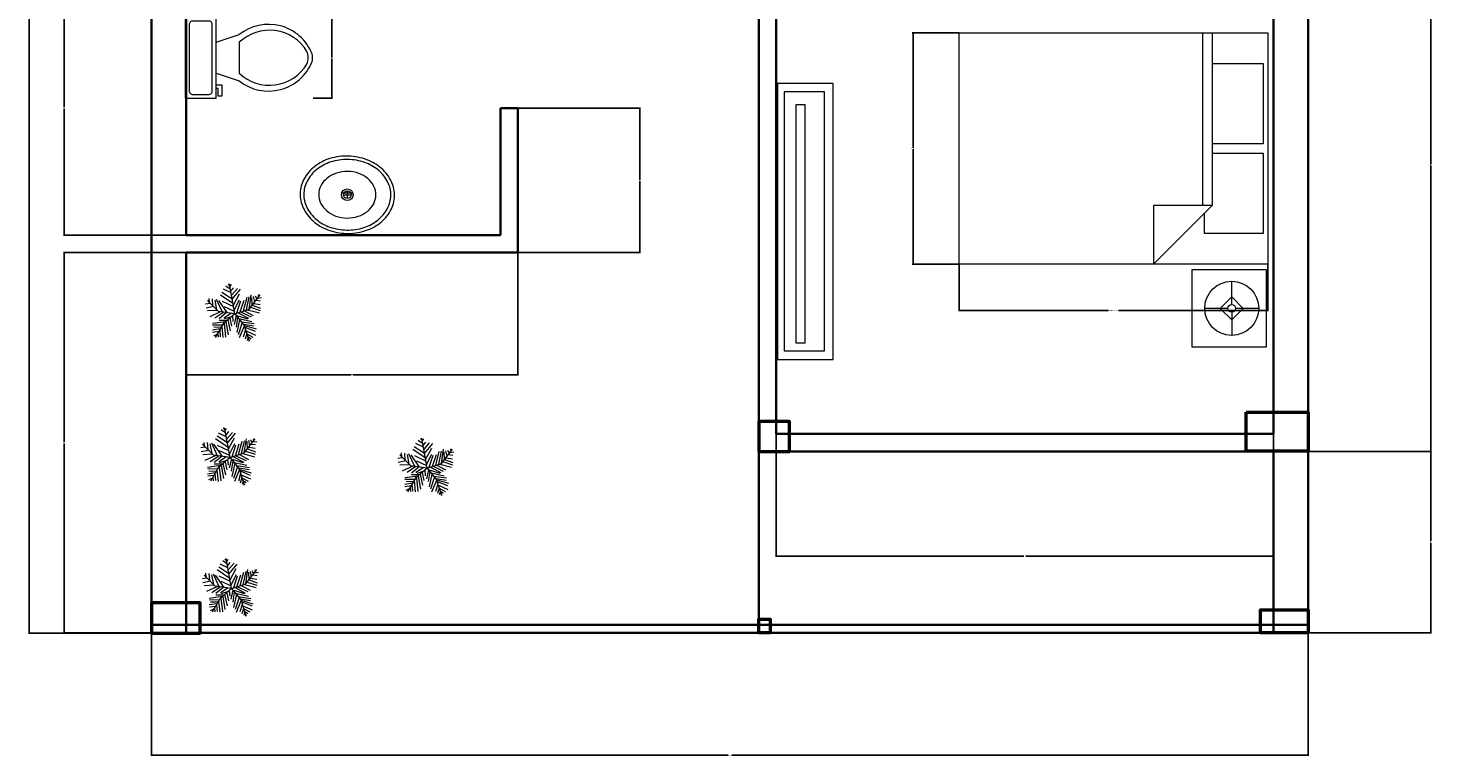
# Model space of a CAD drawing. Units: inches. Extents: x 50 to 2003, y -28 to 675.
# Tile 5 of 10: x 592 to 956, y -28 to 160. Entities that reach past the tile are written whole.
import ezdxf

# ---------------------------------------------------------------- set-up
doc = ezdxf.new("R2010")
doc.units = ezdxf.units.IN
for name, color, linetype, lineweight in [('A-ANNO-DIMS', 2, 'Continuous', 18), ('A-COLS', 1, 'Continuous', 50), ('A-FLOR-FIXT', 9, 'Continuous', 18), ('A-FURN', 8, 'Continuous', 18), ('A-FURN-LITE', 9, 'Continuous', 13), ('A-WALL', 7, 'Continuous', 35), ('L-PLNT', 3, 'Continuous', 13)]:
    doc.layers.add(name, color=color, linetype=linetype, lineweight=lineweight)
doc.styles.get("Standard").update_dxf_attribs({"font": 'arial.ttf'})
doc.dimstyles.get("Standard").update_dxf_attribs({"dimtxt": 0.18, "dimasz": 0.18, "dimexe": 0.18, "dimexo": 0.0625, "dimgap": 0.09, "dimtad": 0, "dimtih": 1, "dimtoh": 1, "dimdec": 4, "dimzin": 0, "dimdsep": 46, "dimtxsty": 'Standard', "dimcen": 0.09, "dimadec": 0, "dimazin": 0, "dimtfac": 1, "dimtdec": 4, "dimtofl": 0, "dimtmove": 0, "dimatfit": 3, "dimfxl": 1, "dimtolj": 1, "dimtzin": 0, "dimarcsym": 0})

# ---------------------------------------------------------------- blocks, each defined once
blk = doc.blocks.new('*U2')
for p, q in [((-10.186, 53.64), (-13.084, 55.962)), ((0, 0), (-10.5, 57)), ((-9.099, 51.782), (-6.563, 55.962)), ((-48.585, 21.131), (-49.309, 29.026)), ((-43.513, 28.561), (-42.427, 15.558)), ((-35.544, 28.097), (-24.314, 3.947)), ((-3.665, 19.273), (-27.574, 35.527)), ((-5.114, 28.097), (-24.676, 40.636)), ((-7.288, 39.707), (-21.778, 46.673)), ((-8.737, 47.138), (-17.069, 52.711)), ((-7.65, 43.423), (-2.578, 49.46)), ((-5.839, 35.992), (4.667, 48.067)), ((-5.114, 27.632), (10.463, 46.673)), ((-2.941, 16.486), (8.652, 37.85)), ((16.259, 5.805), (23.142, 31.348)), ((22.055, 7.198), (27.489, 32.277)), ((27, 9), (48, 36)), ((27.127, 9.056), (31.112, 35.992)), ((31.836, 30.883), (32.561, 16.486)), ((35.096, 32.741), (37.27, 22.524)), ((38.719, 34.134), (41.979, 28.561)), ((43.791, 29.954), (51.036, 30.883)), ((44.153, 36.456), (45.239, 32.741)), ((-47.498, 19.737), (-55.83, 18.344)), ((-40.615, 13.7), (-55.105, 10.913)), ((-31.5, 4.5), (-52.5, 25.5)), ((-33.37, 6.269), (-52.207, 5.34)), ((-28.299, 3.483), (-47.86, -5.805)), ((-38.442, 26.239), (-34.819, 7.663)), ((-21.416, 3.018), (-38.079, -8.128)), ((0, 0), (-31.5, 4.5)), ((-14.533, 2.09), (-30.834, 25.31)), ((-15.982, 2.09), (-30.11, -9.521)), ((-24.314, 23.917), (-2.941, 13.7)), ((0, 0), (-22.5, -19.5)), ((-6.563, 1.161), (-21.416, -8.128)), ((-20.691, 13.7), (-1.129, 4.876)), ((-1.129, 6.734), (9.014, 26.704)), ((0, 0), (27, 9)), ((0, 0), (18, -22.5)), ((3.942, 1.625), (11.187, 24.381)), ((6.478, 1.625), (26.04, -8.592)), ((10.101, 3.483), (17.708, 26.239)), ((11.187, 3.483), (30.749, -5.805)), ((18.07, 5.805), (35.096, -3.483)), ((24.229, 7.663), (46.688, 1.625)), ((29.662, 12.307), (48.137, 6.269)), ((33.285, 16.486), (48.862, 10.913)), ((36.183, 19.737), (48.137, 17.88)), ((40.53, 25.775), (48.862, 24.846)), ((-17.431, -15.094), (-42.789, -18.809)), ((-24.314, -21.596), (-42.427, -22.06)), ((-26.849, -26.24), (-40.253, -25.775)), ((-22.5, -19.5), (-37.5, -45)), ((-15.257, -12.772), (-30.11, -12.772)), ((-25.038, -23.918), (-22.865, -45.281)), ((-20.691, -18.345), (-17.793, -44.352)), ((-6.563, -5.805), (-19.967, -9.985)), ((-17.069, -15.094), (-12.721, -40.172)), ((-13.446, -11.378), (-8.737, -32.741)), ((-9.461, -8.592), (-6.201, -23.453)), ((-4.752, -3.483), (-3.665, -14.629)), ((2.493, -3.019), (-1.491, -20.202)), ((1.769, -2.555), (24.229, -9.521)), ((5.029, -6.27), (2.131, -25.775)), ((9.014, -11.378), (3.58, -35.992)), ((14.085, -16.951), (6.478, -40.172)), ((7.565, -9.056), (32.198, -14.629)), ((18.07, -22.524), (8.289, -45.745)), ((12.274, -15.094), (36.907, -18.809)), ((16.259, -19.738), (36.183, -22.989)), ((18, -22.5), (27, -52.5)), ((18.433, -22.524), (40.53, -29.026)), ((19.157, -25.311), (38.719, -33.206)), ((-28.299, -29.026), (-42.789, -31.348)), ((-30.834, -34.135), (-42.427, -35.528)), ((-34.457, -39.708), (-40.978, -42.494)), ((-32.646, -36.921), (-31.921, -44.352)), ((-29.023, -30.884), (-27.936, -43.887)), ((20.244, -30.419), (15.897, -44.816)), ((22.78, -37.85), (19.519, -48.532)), ((21.331, -32.741), (39.081, -40.636)), ((22.78, -38.314), (34.372, -44.816)), ((24.591, -45.745), (23.142, -50.854)), ((24.591, -43.423), (30.749, -47.603)), ((26.764, -49.925), (28.213, -50.854))]:
    blk.add_line(p, q)
blk = doc.blocks.new('Bed - Queen')
for p, q in [((0, -80.00003), (0, 0)), ((0, 0), (59.99999, 0)), ((59.99999, 0), (59.99999, -80.00003)), ((7.99999, -1.2), (28.79998, -1.2)), ((7.99999, -14.4), (7.99999, -1.2)), ((28.79998, -1.2), (28.79998, -14.4)), ((31.19999, -1.2), (51.99999, -1.2)), ((31.19999, -14.4), (31.19999, -1.2)), ((51.99999, -1.2), (51.99999, -16.4)), ((0, -14.4), (44.8, -14.4)), ((59.99999, -29.6), (44.8, -14.4)), ((44.8, -14.4), (44.8, -29.6)), ((44.8, -16.8), (0, -16.8)), ((51.99999, -16.4), (46.79936, -16.4)), ((44.8, -29.6), (59.99999, -29.6)), ((59.99999, -80.00003), (0, -80.00003))]:
    blk.add_line(p, q)
blk = doc.blocks.new('Lamp - Table')
for p, q in [((0, 7), (0, 1)), ((-1, 0), (-7, 0)), ((0, 3), (-3, 0)), ((-3, 0), (0, -3)), ((3, 0), (0, 3)), ((0, -3), (3, 0)), ((1, 0), (7, 0)), ((0, -1), (0, -7))]:
    blk.add_line(p, q)
for radius in [7, 1]:
    blk.add_circle((0, 0), radius)
blk = doc.blocks.new('Toilet - top')
for p, q in [((9.5, -6), (9.5, -2)), ((-10, -8.5), (-8, -8.5)), ((-10, -9.5), (-10, -8.5)), ((-7, -9.5), (-10, -9.5)), ((-8, -8.5), (-8, -8)), ((-7, -8), (-7, -9.5)), ((-4, -8), (-6, -14)), ((4, -8), (6, -14)), ((4, -14), (-4, -14))]:
    blk.add_line(p, q)
blk.add_lwpolyline([(10.5, -8), (10.5, 0), (-10.5, 0), (-10.5, -8)], close=True)
for points in [[(-9.5, -2), (-9.5, -6)], [(8.5, -1), (-8.5, -1)], [(-8.5, -7), (8.5, -7)]]:
    blk.add_lwpolyline(points)
for centre, radius, start, end in [((-8.62, -1.88), 0.884, 81.8699, 188.1301), ((8.62, -1.88), 0.884, 351.8699, 98.1301), ((-8.62, -6.12), 0.884, 171.8699, 278.1301), ((8.62, -6.12), 0.884, 261.8699, 8.1301), ((3.52, -21.58), 12.17, 141.4691, 247.9714), ((4.2, -21.82), 11.33, 136.3677, 238.9468), ((-3.52, -21.58), 12.17, 292.0284, 38.5307), ((-4.2, -21.82), 11.33, 301.053, 43.6321), ((0, -27.88), 4, 245.7318, 294.2682), ((0, -29), 4, 254.8605, 285.1395)]:
    blk.add_arc(centre, radius, start, end)
blk = doc.blocks.new('Sink - Oval top')
for p, q in [((-1, 0), (1, 0)), ((0, 1), (0, -1))]:
    blk.add_line(p, q)
for points in [[(-12.23, 0.39, 0.117634), (-11.46, -3.36, 0.104469), (-8.88, -6.8, 0.090016), (-5.08, -9.07, 0.08192), (-0.32, -10.02, 0.08192), (4.49, -9.38, 0.090016), (8.42, -7.36, 0.104469), (11.22, -4.09, 0.117634), (12.23, -0.39, 0.117634), (11.46, 3.36, 0.104469), (8.88, 6.8, 0.090016), (5.08, 9.07, 0.08192), (0.32, 10.02, 0.08192), (-4.49, 9.38, 0.090016), (-8.42, 7.36, 0.104469), (-11.22, 4.09, 0.117634)], [(-11.29, 0.16, 0.118622), (-10.52, -3.25, 0.104678), (-8.07, -6.36, 0.089562), (-4.54, -8.37, 0.081185), (-0.13, -9.15, 0.081185), (4.3, -8.49, 0.089562), (7.89, -6.58, 0.104678), (10.42, -3.55, 0.118622), (11.29, -0.16, 0.118622), (10.52, 3.25, 0.104678), (8.07, 6.36, 0.089562), (4.54, 8.37, 0.081185), (0.13, 9.15, 0.081185), (-4.3, 8.49, 0.089562), (-7.89, 6.58, 0.104678), (-10.42, 3.55, 0.118622)], [(-7.42, 0.08, 0.118283), (-6.91, -2.17, 0.104607), (-5.29, -4.21, 0.089718), (-2.97, -5.53, 0.081436), (-0.07, -6.04, 0.081436), (2.84, -5.59, 0.089718), (5.2, -4.33, 0.104607), (6.86, -2.32, 0.118283), (7.42, -0.08, 0.118283), (6.91, 2.17, 0.104607), (5.29, 4.21, 0.089718), (2.97, 5.53, 0.081436), (0.07, 6.04, 0.081436), (-2.84, 5.59, 0.089718), (-5.2, 4.33, 0.104607), (-6.86, 2.32, 0.118283)]]:
    blk.add_lwpolyline(points, format="xyb", close=True)
for radius in [1.5, 1]:
    blk.add_circle((0, 0), radius)
blk = doc.blocks.new('MEDIA-CONSOLE')
for points in [[(0, 0), (71.49, 0), (71.49, 14.4), (0, 14.4)], [(2.13, 1.7), (69.3, 1.7), (69.3, 12.15), (2.13, 12.15)], [(5.56, 4.74), (67.2, 4.74), (67.2, 7.16), (5.56, 7.16)]]:
    blk.add_lwpolyline(points, close=True)
blk = doc.blocks.new('NIGHTSTAND-STANDARD')
blk.add_lwpolyline([(0, 0), (0, 20.13), (19.19, 20.13), (19.19, 0)], close=True)
blk = doc.blocks.new('*D23')
at = {"layer": 'A-ANNO-DIMS', "color": 0, "lineweight": -2, "transparency": 16777216}
for p, q in [((833.11, 99.05), (833.11, 86.94)), ((913.11, 99.05), (913.11, 86.94)), ((833.29, 87.12), (871.8, 87.12)), ((912.93, 87.12), (874.41, 87.12))]:
    blk.add_line(p, q, dxfattribs=at)
at = {"layer": 'A-ANNO-DIMS', "color": 0, "transparency": 16777216}
for points in [[(833.29, 87.15), (833.29, 87.09), (833.11, 87.12)], [(912.93, 87.15), (912.93, 87.09), (913.11, 87.12)]]:
    blk.add_solid(points, dxfattribs=at)
at = {"layer": 'Defpoints', "color": 0, "transparency": 16777216}
for p in [(833.11, 99.12), (913.11, 99.12), (913.11, 87.12)]:
    blk.add_point(p, dxfattribs=at)
at = {"layer": 'A-ANNO-DIMS', "color": 0, "transparency": 16777216, "insert": (873.11, 87.12), "char_height": 0.18, "attachment_point": 5}
blk.add_mtext('\\A1;QUEEN BED 80 TYP.', dxfattribs=at)
blk = doc.blocks.new('*D24')
at = {"layer": 'A-ANNO-DIMS', "color": 0, "lineweight": -2, "transparency": 16777216}
for p, q in [((833.04, 159.12), (820.93, 159.12)), ((821.11, 158.94), (821.11, 129.3)), ((821.11, 99.3), (821.11, 128.93)), ((833.04, 99.12), (820.93, 99.12))]:
    blk.add_line(p, q, dxfattribs=at)
at = {"layer": 'A-ANNO-DIMS', "color": 0, "transparency": 16777216}
for points in [[(821.08, 158.94), (821.14, 158.94), (821.11, 159.12)], [(821.08, 99.3), (821.14, 99.3), (821.11, 99.12)]]:
    blk.add_solid(points, dxfattribs=at)
at = {"layer": 'Defpoints', "color": 0, "transparency": 16777216}
for p in [(833.11, 159.12), (821.11, 99.12), (833.11, 99.12)]:
    blk.add_point(p, dxfattribs=at)
at = {"layer": 'A-ANNO-DIMS', "color": 0, "transparency": 16777216, "insert": (821.11, 129.12), "char_height": 0.18, "attachment_point": 5}
blk.add_mtext('\\A1;60 TYP.', dxfattribs=at)
blk = doc.blocks.new('*D30')
at = {"layer": 'A-ANNO-DIMS', "color": 0, "lineweight": -2, "transparency": 16777216}
for p, q in [((665.51, 163.13), (670.58, 163.13)), ((670.4, 162.95), (670.4, 152.81)), ((670.4, 142.31), (670.4, 152.45)), ((665.51, 142.13), (670.58, 142.13))]:
    blk.add_line(p, q, dxfattribs=at)
at = {"layer": 'A-ANNO-DIMS', "color": 0, "transparency": 16777216}
for points in [[(670.37, 162.95), (670.43, 162.95), (670.4, 163.13)], [(670.37, 142.31), (670.43, 142.31), (670.4, 142.13)]]:
    blk.add_solid(points, dxfattribs=at)
at = {"layer": 'Defpoints', "color": 0, "transparency": 16777216}
for p in [(665.44, 163.13), (670.4, 163.13), (665.44, 142.13)]:
    blk.add_point(p, dxfattribs=at)
at = {"layer": 'A-ANNO-DIMS', "color": 0, "transparency": 16777216, "insert": (670.4, 152.63), "char_height": 0.18, "attachment_point": 5}
blk.add_mtext('\\A1;21 TYP.', dxfattribs=at)
blk = doc.blocks.new('*D74')
at = {"layer": 'A-ANNO-DIMS', "color": 0, "lineweight": -2, "transparency": 16777216}
for p, q in [((623.65, 3.46), (623.65, -28.31)), ((923.6, 3.56), (923.6, -28.31)), ((623.83, -28.13), (773.16, -28.13)), ((923.42, -28.13), (774.09, -28.13))]:
    blk.add_line(p, q, dxfattribs=at)
at = {"layer": 'A-ANNO-DIMS', "color": 0, "transparency": 16777216}
for points in [[(623.83, -28.1), (623.83, -28.16), (623.65, -28.13)], [(923.42, -28.1), (923.42, -28.16), (923.6, -28.13)]]:
    blk.add_solid(points, dxfattribs=at)
at = {"layer": 'Defpoints', "color": 0, "transparency": 16777216}
for p in [(623.65, 3.52), (923.6, 3.62), (923.6, -28.13)]:
    blk.add_point(p, dxfattribs=at)
at = {"layer": 'A-ANNO-DIMS', "color": 0, "transparency": 16777216, "insert": (773.63, -28.13), "char_height": 0.18, "attachment_point": 5}
blk.add_mtext('\\A1;299.95', dxfattribs=at)
blk = doc.blocks.new('*D75')
at = {"layer": 'A-ANNO-DIMS', "color": 0, "lineweight": -2, "transparency": 16777216}
for p, q in [((623.55, 618.62), (591.74, 618.62)), ((591.92, 618.44), (591.92, 311.25)), ((591.92, 3.7), (591.92, 310.89)), ((623.59, 3.52), (591.74, 3.52))]:
    blk.add_line(p, q, dxfattribs=at)
at = {"layer": 'A-ANNO-DIMS', "color": 0, "transparency": 16777216}
for points in [[(591.89, 618.44), (591.95, 618.44), (591.92, 618.62)], [(591.89, 3.7), (591.95, 3.7), (591.92, 3.52)]]:
    blk.add_solid(points, dxfattribs=at)
at = {"layer": 'Defpoints', "color": 0, "transparency": 16777216}
for p in [(591.92, 618.62), (623.62, 618.62), (623.65, 3.52)]:
    blk.add_point(p, dxfattribs=at)
at = {"layer": 'A-ANNO-DIMS', "color": 0, "transparency": 16777216, "insert": (591.92, 311.07), "char_height": 0.18, "attachment_point": 5}
blk.add_mtext('\\A1;615.1', dxfattribs=at)
blk = doc.blocks.new('*D76')
at = {"layer": 'A-ANNO-DIMS', "color": 0, "lineweight": -2, "transparency": 16777216}
for p, q in [((785.62, 55.06), (785.62, 23.29)), ((914.62, 55.06), (914.62, 23.29)), ((785.8, 23.47), (849.84, 23.47)), ((914.44, 23.47), (850.4, 23.47))]:
    blk.add_line(p, q, dxfattribs=at)
at = {"layer": 'A-ANNO-DIMS', "color": 0, "transparency": 16777216}
for points in [[(785.8, 23.5), (785.8, 23.44), (785.62, 23.47)], [(914.44, 23.5), (914.44, 23.44), (914.62, 23.47)]]:
    blk.add_solid(points, dxfattribs=at)
at = {"layer": 'Defpoints', "color": 0, "transparency": 16777216}
for p in [(785.62, 55.12), (914.62, 55.12), (785.62, 23.47)]:
    blk.add_point(p, dxfattribs=at)
at = {"layer": 'A-ANNO-DIMS', "color": 0, "transparency": 16777216, "insert": (850.12, 23.47), "char_height": 0.18, "attachment_point": 5}
blk.add_mtext('\\A1;129', dxfattribs=at)
blk = doc.blocks.new('*D80')
at = {"layer": 'A-ANNO-DIMS', "color": 0, "lineweight": -2, "transparency": 16777216}
for p, q in [((914.678813, 50.62165), (955.559258, 50.62165)), ((955.379258, 50.44165), (955.379258, 27.30165)), ((955.379258, 3.80165), (955.379258, 26.94165)), ((923.678813, 3.62165), (955.559258, 3.62165))]:
    blk.add_line(p, q, dxfattribs=at)
at = {"layer": 'A-ANNO-DIMS', "color": 0, "transparency": 16777216}
for points in [[(955.349258, 50.44165), (955.409258, 50.44165), (955.379258, 50.62165)], [(955.349258, 3.80165), (955.409258, 3.80165), (955.379258, 3.62165)]]:
    blk.add_solid(points, dxfattribs=at)
at = {"layer": 'Defpoints', "color": 0, "transparency": 16777216}
for p in [(914.616313, 50.62165), (955.379258, 50.62165), (923.616313, 3.62165)]:
    blk.add_point(p, dxfattribs=at)
at = {"layer": 'A-ANNO-DIMS', "color": 0, "transparency": 16777216, "insert": (955.379258, 27.12165), "char_height": 0.18, "attachment_point": 5}
blk.add_mtext('\\A1;47', dxfattribs=at)
blk = doc.blocks.new('*D81')
at = {"layer": 'A-ANNO-DIMS', "color": 0, "lineweight": -2, "transparency": 16777216}
for p, q in [((914.68, 199.12), (955.56, 199.12)), ((955.38, 198.94), (955.38, 125.05)), ((955.38, 50.8), (955.38, 124.69)), ((914.68, 50.62), (955.56, 50.62))]:
    blk.add_line(p, q, dxfattribs=at)
at = {"layer": 'A-ANNO-DIMS', "color": 0, "transparency": 16777216}
for points in [[(955.35, 198.94), (955.41, 198.94), (955.38, 199.12)], [(955.35, 50.8), (955.41, 50.8), (955.38, 50.62)]]:
    blk.add_solid(points, dxfattribs=at)
at = {"layer": 'Defpoints', "color": 0, "transparency": 16777216}
for p in [(914.62, 199.12), (955.38, 199.12), (914.62, 50.62)]:
    blk.add_point(p, dxfattribs=at)
at = {"layer": 'A-ANNO-DIMS', "color": 0, "transparency": 16777216, "insert": (955.38, 124.87), "char_height": 0.18, "attachment_point": 5}
blk.add_mtext('\\A1;148.5', dxfattribs=at)
blk = doc.blocks.new('*D85')
at = {"layer": 'A-ANNO-DIMS', "color": 0, "lineweight": -2, "transparency": 16777216}
for p, q in [((632.55, 102.12), (600.79, 102.12)), ((600.97, 101.94), (600.97, 53.05)), ((600.97, 3.8), (600.97, 52.69)), ((632.55, 3.62), (600.79, 3.62))]:
    blk.add_line(p, q, dxfattribs=at)
at = {"layer": 'A-ANNO-DIMS', "color": 0, "transparency": 16777216}
for points in [[(600.94, 101.94), (601, 101.94), (600.97, 102.12)], [(600.94, 3.8), (601, 3.8), (600.97, 3.62)]]:
    blk.add_solid(points, dxfattribs=at)
at = {"layer": 'Defpoints', "color": 0, "transparency": 16777216}
for p in [(600.97, 102.12), (632.62, 102.12), (632.62, 3.62)]:
    blk.add_point(p, dxfattribs=at)
at = {"layer": 'A-ANNO-DIMS', "color": 0, "transparency": 16777216, "insert": (600.97, 52.87), "char_height": 0.18, "attachment_point": 5}
blk.add_mtext('\\A1;98.5', dxfattribs=at)
blk = doc.blocks.new('*D86')
at = {"layer": 'A-ANNO-DIMS', "color": 0, "lineweight": -2, "transparency": 16777216}
for p, q in [((632.55, 172.62), (600.79, 172.62)), ((600.97, 172.44), (600.97, 139.8)), ((600.97, 106.8), (600.97, 139.44)), ((632.55, 106.62), (600.79, 106.62))]:
    blk.add_line(p, q, dxfattribs=at)
at = {"layer": 'A-ANNO-DIMS', "color": 0, "transparency": 16777216}
for points in [[(600.94, 172.44), (601, 172.44), (600.97, 172.62)], [(600.94, 106.8), (601, 106.8), (600.97, 106.62)]]:
    blk.add_solid(points, dxfattribs=at)
at = {"layer": 'Defpoints', "color": 0, "transparency": 16777216}
for p in [(600.97, 172.62), (632.62, 172.62), (632.62, 106.62)]:
    blk.add_point(p, dxfattribs=at)
at = {"layer": 'A-ANNO-DIMS', "color": 0, "transparency": 16777216, "insert": (600.97, 139.62), "char_height": 0.18, "attachment_point": 5}
blk.add_mtext('\\A1;66', dxfattribs=at)
blk = doc.blocks.new('*D88')
at = {"layer": 'A-ANNO-DIMS', "color": 0, "lineweight": -2, "transparency": 16777216}
for p, q in [((632.62, 102.06), (632.62, 70.29)), ((718.62, 102.06), (718.62, 70.29)), ((632.8, 70.47), (675.4, 70.47)), ((718.44, 70.47), (675.84, 70.47))]:
    blk.add_line(p, q, dxfattribs=at)
at = {"layer": 'A-ANNO-DIMS', "color": 0, "transparency": 16777216}
for points in [[(632.8, 70.5), (632.8, 70.44), (632.62, 70.47)], [(718.44, 70.5), (718.44, 70.44), (718.62, 70.47)]]:
    blk.add_solid(points, dxfattribs=at)
at = {"layer": 'Defpoints', "color": 0, "transparency": 16777216}
for p in [(632.62, 102.12), (718.62, 102.12), (632.62, 70.47)]:
    blk.add_point(p, dxfattribs=at)
at = {"layer": 'A-ANNO-DIMS', "color": 0, "transparency": 16777216, "insert": (675.62, 70.47), "char_height": 0.18, "attachment_point": 5}
blk.add_mtext('\\A1;86', dxfattribs=at)
blk = doc.blocks.new('*D89')
at = {"layer": 'A-ANNO-DIMS', "color": 0, "lineweight": -2, "transparency": 16777216}
for p, q in [((718.68, 139.56), (750.45, 139.56)), ((750.27, 139.38), (750.27, 121.02)), ((750.27, 102.3), (750.27, 120.66)), ((718.68, 102.12), (750.45, 102.12))]:
    blk.add_line(p, q, dxfattribs=at)
at = {"layer": 'A-ANNO-DIMS', "color": 0, "transparency": 16777216}
for points in [[(750.24, 139.38), (750.3, 139.38), (750.27, 139.56)], [(750.24, 102.3), (750.3, 102.3), (750.27, 102.12)]]:
    blk.add_solid(points, dxfattribs=at)
at = {"layer": 'Defpoints', "color": 0, "transparency": 16777216}
for p in [(718.62, 139.56), (718.62, 102.12), (750.27, 102.12)]:
    blk.add_point(p, dxfattribs=at)
at = {"layer": 'A-ANNO-DIMS', "color": 0, "transparency": 16777216, "insert": (750.27, 120.84), "char_height": 0.18, "attachment_point": 5}
blk.add_mtext('\\A1;37.435', dxfattribs=at)

msp = doc.modelspace()

# ---------------------------------------------------------------- linework, layer by layer
at = {"layer": 'A-COLS'}
for points in [[(781.114, 50.5781), (789.1039, 50.5781), (789.1039, 58.3676), (781.114, 58.3676)], [(907.5433, 60.7944), (923.6157, 60.7944), (923.6157, 50.6622), (907.5433, 50.6622)], [(623.6536, 3.5196), (636.2297, 3.5196), (636.2297, 11.3747), (623.6536, 11.3747)], [(923.6009, 3.6211), (911.2482, 3.6211), (911.2482, 9.5147), (923.6009, 9.5147)], [(781.0669, 3.6558), (784.1128, 3.6558), (784.1128, 7.0467), (781.0669, 7.0467)]]:
    msp.add_lwpolyline(points, close=True, dxfattribs=at)
at = {"layer": 'A-FLOR-FIXT'}
msp.add_line((672.9803, 117.5999), (675.8206, 117.5999), dxfattribs=at)
at = {"layer": 'A-WALL'}
for p, q in [((623.6163, 3.6216), (623.6163, 618.6217)), ((923.6163, 618.6217), (923.6163, 3.6216)), ((781.1163, 3.6216), (781.1163, 203.6217)), ((785.6163, 55.1217), (785.6163, 199.1216)), ((914.6163, 199.1216), (914.6163, 55.1217)), ((632.6163, 106.6217), (632.6163, 172.6216)), ((714.1163, 106.6217), (714.1163, 139.5565)), ((714.1163, 139.5565), (718.6163, 139.5565)), ((718.6163, 102.1217), (718.6163, 139.5565)), ((632.6163, 106.6217), (714.1163, 106.6217)), ((632.6163, 3.6216), (632.6163, 102.1217)), ((632.6163, 102.1217), (718.6163, 102.1217)), ((785.6163, 55.1217), (914.6163, 55.1217)), ((781.1163, 50.6217), (914.6163, 50.6217)), ((914.6163, 50.6217), (914.6163, 3.6216)), ((623.6163, 5.6217), (923.6163, 5.6217)), ((623.6163, 3.6216), (923.6163, 3.6216))]:
    msp.add_line(p, q, dxfattribs=at)

# ---------------------------------------------------------------- block references
at = {"layer": 'A-FLOR-FIXT', "rotation": 89.99999999999999}
msp.add_blockref('Toilet - top', (632.3978, 152.6305), dxfattribs=at)
at = {"layer": 'A-FLOR-FIXT'}
msp.add_blockref('Sink - Oval top', (674.4004, 117.1169), dxfattribs=at)
at = {"layer": 'A-FURN'}
for name, p, rotation in [('Bed - Queen', (913.1075, 159.1164), 270), ('MEDIA-CONSOLE', (785.9959, 145.9394), 269.9999999999996), ('NIGHTSTAND-STANDARD', (912.7138, 97.7628), 180)]:
    msp.add_blockref(name, p, dxfattribs=dict(at, rotation=rotation))
at = {"layer": 'A-FURN-LITE', "rotation": 270}
msp.add_blockref('Lamp - Table', (903.7721, 87.6807), dxfattribs=at)
at = {"layer": 'L-PLNT', "xscale": 0.1358686367750108, "yscale": 0.1358686367750108, "zscale": 0.1358686367750108}
for p in [(645.2512, 86.2759), (643.9939, 48.9991), (695.1245, 46.2767), (644.413, 15.073)]:
    msp.add_blockref('*U2', p, dxfattribs=at)

# ---------------------------------------------------------------- dimensions: what is measured, and where the dimension line sits
at = {"layer": 'A-ANNO-DIMS'}
for base, p1, p2, angle, override, picture, middle in [((591.9232, 618.6217), (623.6536, 3.5196), (623.6163, 618.6217), 90, {"dimdec": 1, "dimlfac": 1, "dimrnd": 0, "dimzin": 0, "dimdsep": 46, "dimlunit": 2}, '*D75', (591.9232, 311.0706)), ((955.3793, 199.1216), (914.6163, 50.6217), (914.6163, 199.1216), 90, {"dimdec": 1, "dimlfac": 1, "dimrnd": 0, "dimzin": 0, "dimdsep": 46, "dimlunit": 2}, '*D81', (955.3793, 124.8716)), ((600.9663, 172.6216), (632.6163, 106.6217), (632.6163, 172.6216), 90, {"dimdec": 0, "dimlfac": 1, "dimrnd": 0, "dimzin": 0, "dimdsep": 46, "dimlunit": 2}, '*D86', (600.9663, 139.6216)), ((750.2663, 102.1217), (718.6163, 139.5565), (718.6163, 102.1217), 270, {"dimdec": 3, "dimlfac": 1, "dimrnd": 0, "dimzin": 0, "dimdsep": 46, "dimlunit": 2}, '*D89', (750.2663, 120.8391)), ((600.9663, 102.1217), (632.6163, 3.6216), (632.6163, 102.1217), 90, {"dimdec": 1, "dimlfac": 1, "dimrnd": 0, "dimzin": 0, "dimdsep": 46, "dimlunit": 2}, '*D85', (600.9663, 52.8716)), ((632.6163, 70.4716), (718.6163, 102.1217), (632.6163, 102.1217), 180, {"dimdec": 0, "dimlfac": 1, "dimrnd": 0, "dimzin": 0, "dimdsep": 46, "dimlunit": 2}, '*D88', (675.6163, 70.4716)), ((785.6163, 23.4717), (914.6163, 55.1217), (785.6163, 55.1217), 180, {"dimdec": 0, "dimlfac": 1, "dimrnd": 0, "dimzin": 0, "dimdsep": 46, "dimlunit": 2}, '*D76', (850.1163, 23.4717)), ((955.3793, 50.6217), (923.6163, 3.6216), (914.6163, 50.6217), 90, {"dimdec": 0, "dimlfac": 1, "dimrnd": 0, "dimzin": 0, "dimdsep": 46, "dimlunit": 2}, '*D80', (955.3793, 27.1216))]:
    dim = msp.add_linear_dim(base=base, p1=p1, p2=p2, angle=angle, dimstyle='Standard', override=override, dxfattribs=at)
    dim.commit()
    dim.dimension.update_dxf_attribs({"geometry": picture, "text_midpoint": middle})
for base, p1, p2, angle, picture, middle in [((670.401, 163.1305), (665.4441, 142.1305), (665.4441, 163.1305), 90, '*D30', (670.401, 152.6305)), ((821.1075, 99.1165), (833.1075, 159.1164), (833.1075, 99.1165), 270, '*D24', (821.1075, 129.1165))]:
    dim = msp.add_linear_dim(base=base, p1=p1, p2=p2, angle=angle, text='<> TYP.', dimstyle='Standard', override={"dimdec": 0, "dimlfac": 1, "dimrnd": 0, "dimzin": 0, "dimdsep": 46, "dimlunit": 2}, dxfattribs=at)
    dim.commit()
    dim.dimension.update_dxf_attribs({"geometry": picture, "text_midpoint": middle})
dim = msp.add_linear_dim(base=(913.1075, 87.1165), p1=(833.1075, 99.1165), p2=(913.1075, 99.1165), text='QUEEN BED <> TYP.', dimstyle='Standard', override={"dimdec": 0, "dimlfac": 1, "dimrnd": 0, "dimzin": 0, "dimdsep": 46, "dimlunit": 2}, dxfattribs=at)
dim.commit()
dim.dimension.update_dxf_attribs({"geometry": '*D23', "text_midpoint": (873.1075, 87.1165)})
dim = msp.add_linear_dim(base=(923.6009, -28.1304), p1=(623.6536, 3.5196), p2=(923.6009, 3.6211), dimstyle='Standard', override={"dimdec": 2, "dimlfac": 1, "dimrnd": 0, "dimzin": 0, "dimdsep": 46, "dimlunit": 2}, dxfattribs=at)
dim.commit()
dim.dimension.update_dxf_attribs({"geometry": '*D74', "text_midpoint": (773.6272, -28.1304)})

doc.saveas('drawing.dxf')
